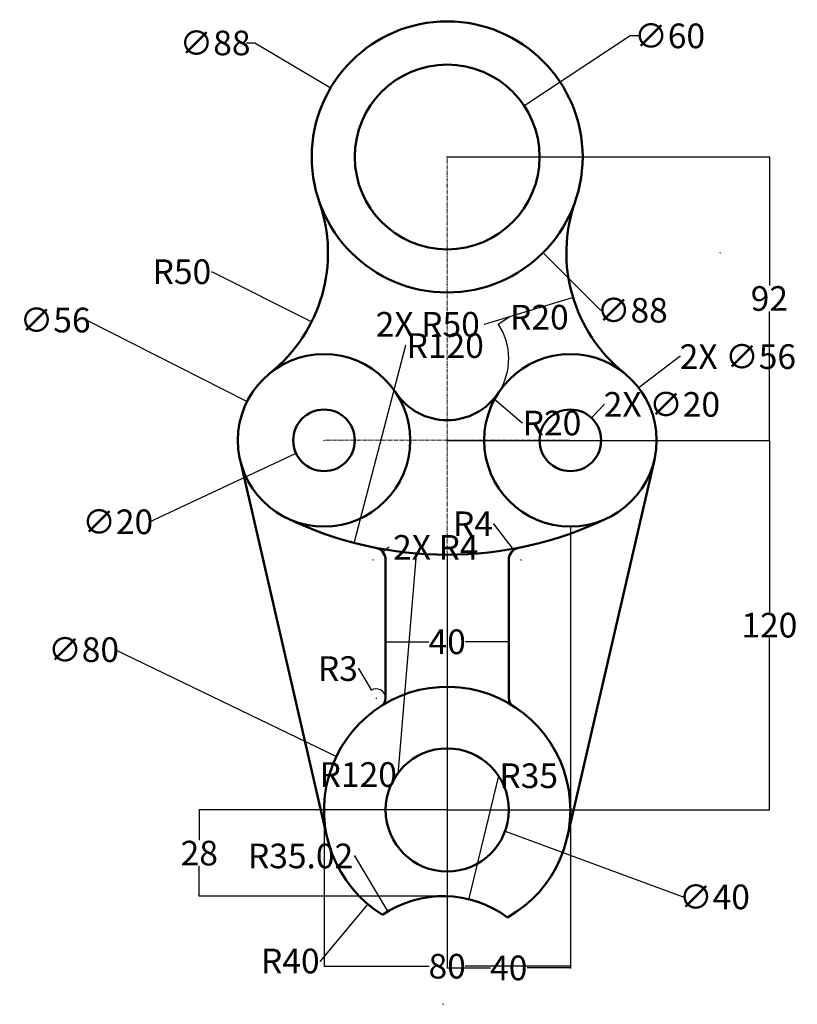
# Model space of a CAD drawing. Units: inches. Extents: x 453 to 706, y -10 to 310.
import ezdxf

# ---------------------------------------------------------------- set-up
doc = ezdxf.new("R2010")
doc.units = ezdxf.units.IN
doc.header["$MEASUREMENT"] = 0
doc.linetypes.add('CENTER', pattern=[2, 1.25, -0.25, 0.25, -0.25])
for name, color, linetype, lineweight in [('M-CNTR', 41, 'CENTER', 18), ('M-CONS', 8, 'Continuous', 13), ('M-DIMS', 131, 'Continuous', 25), ('M-OUTL', 7, 'Continuous', 50)]:
    doc.layers.add(name, color=color, linetype=linetype, lineweight=lineweight)
doc.styles.get("Standard").update_dxf_attribs({"font": 'arial.ttf'})
doc.dimstyles.new('Copy of Standard', dxfattribs={"dimtxt": 8, "dimasz": 0.18, "dimexe": 0.18, "dimexo": 0.0625, "dimgap": 0.09, "dimtad": 0, "dimtih": 1, "dimtoh": 1, "dimdec": 0, "dimzin": 0, "dimdsep": 46, "dimtxsty": 'Standard', "dimcen": 0.09, "dimadec": 0, "dimazin": 0, "dimtfac": 1, "dimtdec": 0, "dimtofl": 0, "dimtmove": 0, "dimatfit": 3, "dimfxl": 1, "dimtolj": 1, "dimtzin": 0, "dimarcsym": 0})

# ---------------------------------------------------------------- blocks, each defined once
blk = doc.blocks.new('*D1')
at = {"layer": 'Defpoints', "color": 0, "transparency": 16777216}
for p in [(554.31, 287.74), (630.03, 242.91)]:
    blk.add_point(p, dxfattribs=at)
at = {"layer": 'M-DIMS', "color": 0, "lineweight": -2, "transparency": 16777216}
for p, q in [((526.97, 302.32), (529.67, 302.32)), ((529.67, 302.32), (554.15, 287.83)), ((592.08, 265.32), (592.26, 265.32)), ((592.17, 265.23), (592.17, 265.41))]:
    blk.add_line(p, q, dxfattribs=at)
at = {"layer": 'M-DIMS', "color": 0, "transparency": 16777216}
blk.add_solid([(554.17, 287.85), (554.14, 287.8), (554.31, 287.74)], dxfattribs=at)
at = {"layer": 'M-DIMS', "color": 0, "transparency": 16777216, "insert": (516.79, 302.32), "char_height": 8, "attachment_point": 5}
blk.add_mtext('\\A1;∅88', dxfattribs=at)
blk = doc.blocks.new('*D2')
at = {"layer": 'Defpoints', "color": 0, "transparency": 16777216}
for p in [(617.19, 281.88), (567.16, 248.76)]:
    blk.add_point(p, dxfattribs=at)
at = {"layer": 'M-DIMS', "color": 0, "lineweight": -2, "transparency": 16777216}
for p, q in [((651.55, 304.63), (617.34, 281.98)), ((654.25, 304.63), (651.55, 304.63)), ((592.08, 265.32), (592.26, 265.32)), ((592.17, 265.23), (592.17, 265.41))]:
    blk.add_line(p, q, dxfattribs=at)
at = {"layer": 'M-DIMS', "color": 0, "transparency": 16777216}
blk.add_solid([(617.32, 282), (617.35, 281.95), (617.19, 281.88)], dxfattribs=at)
at = {"layer": 'M-DIMS', "color": 0, "transparency": 16777216, "insert": (664.41, 304.63), "char_height": 8, "attachment_point": 5}
blk.add_mtext('\\A1;∅60', dxfattribs=at)
blk = doc.blocks.new('*D3')
at = {"layer": 'Defpoints', "color": 0, "transparency": 16777216}
for p in [(503.46, 234.24), (548.18, 211.87)]:
    blk.add_point(p, dxfattribs=at)
at = {"layer": 'M-DIMS', "color": 0, "lineweight": -2, "transparency": 16777216}
for p, q in [((515.64, 228.06), (515.82, 228.06)), ((515.82, 228.06), (548.02, 211.95))]:
    blk.add_line(p, q, dxfattribs=at)
at = {"layer": 'M-DIMS', "color": 0, "transparency": 16777216}
blk.add_solid([(548.03, 211.98), (548, 211.93), (548.18, 211.87)], dxfattribs=at)
at = {"layer": 'M-DIMS', "color": 0, "transparency": 16777216, "insert": (506.01, 228.06), "char_height": 8, "attachment_point": 5}
blk.add_mtext('\\A1;R50', dxfattribs=at)
blk = doc.blocks.new('*D4')
at = {"layer": 'Defpoints', "color": 0, "transparency": 16777216}
for p in [(592.17, 256.17), (561.94, 140.04)]:
    blk.add_point(p, dxfattribs=at)
at = {"layer": 'M-DIMS', "color": 0, "lineweight": -2, "transparency": 16777216}
for p, q in [((578.61, 204.07), (561.99, 140.22)), ((578.79, 204.07), (578.61, 204.07))]:
    blk.add_line(p, q, dxfattribs=at)
at = {"layer": 'M-DIMS', "color": 0, "transparency": 16777216}
blk.add_solid([(561.96, 140.22), (562.01, 140.21), (561.94, 140.04)], dxfattribs=at)
at = {"layer": 'M-DIMS', "color": 0, "transparency": 16777216, "insert": (591.53, 204.07), "char_height": 8, "attachment_point": 5}
blk.add_mtext('\\A1;R120', dxfattribs=at)
blk = doc.blocks.new('*D5')
at = {"layer": 'Defpoints', "color": 0, "transparency": 16777216}
for p in [(608.81, 210.96), (592.17, 199.85)]:
    blk.add_point(p, dxfattribs=at)
at = {"layer": 'M-DIMS', "color": 0, "lineweight": -2, "transparency": 16777216}
for p, q in [((612.31, 213.3), (608.96, 211.06)), ((612.49, 213.3), (612.31, 213.3)), ((592.08, 199.85), (592.26, 199.85)), ((592.17, 199.76), (592.17, 199.94))]:
    blk.add_line(p, q, dxfattribs=at)
blk.add_arc((592.17, 199.85), 20, 326.6217, 34.236, dxfattribs=at)
at = {"layer": 'M-DIMS', "color": 0, "transparency": 16777216}
blk.add_solid([(608.94, 211.08), (608.97, 211.03), (608.81, 210.96)], dxfattribs=at)
at = {"layer": 'M-DIMS', "color": 0, "transparency": 16777216, "insert": (622.12, 213.3), "char_height": 8, "attachment_point": 5}
blk.add_mtext('\\A1;R20', dxfattribs=at)
blk = doc.blocks.new('*D6')
at = {"layer": 'Defpoints', "color": 0, "transparency": 16777216}
for p in [(592.17, 265.41), (592.17, 173.32), (696.8, 173.32)]:
    blk.add_point(p, dxfattribs=at)
at = {"layer": 'M-DIMS', "color": 0, "lineweight": -2, "transparency": 16777216}
for p, q in [((592.23, 265.41), (696.98, 265.41)), ((696.8, 265.23), (696.8, 223.54)), ((696.8, 173.5), (696.8, 215.19)), ((592.23, 173.32), (696.98, 173.32))]:
    blk.add_line(p, q, dxfattribs=at)
at = {"layer": 'M-DIMS', "color": 0, "transparency": 16777216}
for points in [[(696.77, 265.23), (696.83, 265.23), (696.8, 265.41)], [(696.77, 173.5), (696.83, 173.5), (696.8, 173.32)]]:
    blk.add_solid(points, dxfattribs=at)
at = {"layer": 'M-DIMS', "color": 0, "transparency": 16777216, "insert": (696.8, 219.37), "char_height": 8, "attachment_point": 5}
blk.add_mtext('\\A1;92', dxfattribs=at)
blk = doc.blocks.new('*D7')
at = {"layer": 'Defpoints', "color": 0, "transparency": 16777216}
for p in [(592.17, 173.32), (696.8, 173.32), (592.17, 53.32)]:
    blk.add_point(p, dxfattribs=at)
at = {"layer": 'M-DIMS', "color": 0, "lineweight": -2, "transparency": 16777216}
for p, q in [((592.23, 173.32), (696.98, 173.32)), ((696.8, 173.14), (696.8, 117.5)), ((696.8, 53.5), (696.8, 109.15)), ((592.23, 53.32), (696.98, 53.32))]:
    blk.add_line(p, q, dxfattribs=at)
at = {"layer": 'M-DIMS', "color": 0, "transparency": 16777216}
for points in [[(696.77, 173.14), (696.83, 173.14), (696.8, 173.32)], [(696.77, 53.5), (696.83, 53.5), (696.8, 53.32)]]:
    blk.add_solid(points, dxfattribs=at)
at = {"layer": 'M-DIMS', "color": 0, "transparency": 16777216, "insert": (696.8, 113.32), "char_height": 8, "attachment_point": 5}
blk.add_mtext('\\A1;120', dxfattribs=at)
blk = doc.blocks.new('*D8')
at = {"layer": 'Defpoints', "color": 0, "transparency": 16777216}
for p in [(511.67, 53.32), (592.17, 53.32), (592.17, 25.32)]:
    blk.add_point(p, dxfattribs=at)
at = {"layer": 'M-DIMS', "color": 0, "lineweight": -2, "transparency": 16777216}
for p, q in [((592.11, 53.32), (511.49, 53.32)), ((511.67, 53.14), (511.67, 43.5)), ((511.67, 25.5), (511.67, 35.15)), ((592.11, 25.32), (511.49, 25.32))]:
    blk.add_line(p, q, dxfattribs=at)
at = {"layer": 'M-DIMS', "color": 0, "transparency": 16777216}
for points in [[(511.64, 53.14), (511.7, 53.14), (511.67, 53.32)], [(511.64, 25.5), (511.7, 25.5), (511.67, 25.32)]]:
    blk.add_solid(points, dxfattribs=at)
at = {"layer": 'M-DIMS', "color": 0, "transparency": 16777216, "insert": (511.67, 39.32), "char_height": 8, "attachment_point": 5}
blk.add_mtext('\\A1;28', dxfattribs=at)
blk = doc.blocks.new('*D9')
at = {"layer": 'Defpoints', "color": 0, "transparency": 16777216}
for p in [(561.23, 177.55), (543.11, 169.09)]:
    blk.add_point(p, dxfattribs=at)
at = {"layer": 'M-DIMS', "color": 0, "lineweight": -2, "transparency": 16777216}
for p, q in [((552.08, 173.32), (552.26, 173.32)), ((552.17, 173.23), (552.17, 173.41)), ((495.51, 146.87), (542.95, 169.02)), ((495.33, 146.87), (495.51, 146.87))]:
    blk.add_line(p, q, dxfattribs=at)
at = {"layer": 'M-DIMS', "color": 0, "transparency": 16777216}
blk.add_solid([(542.93, 169.04), (542.96, 168.99), (543.11, 169.09)], dxfattribs=at)
at = {"layer": 'M-DIMS', "color": 0, "transparency": 16777216, "insert": (485.17, 146.87), "char_height": 8, "attachment_point": 5}
blk.add_mtext('\\A1;∅20', dxfattribs=at)
blk = doc.blocks.new('*D10')
at = {"layer": 'Defpoints', "color": 0, "transparency": 16777216}
for p in [(527.2, 185.99), (577.14, 160.65)]:
    blk.add_point(p, dxfattribs=at)
at = {"layer": 'M-DIMS', "color": 0, "lineweight": -2, "transparency": 16777216}
for p, q in [((475.01, 212.37), (475.19, 212.37)), ((475.19, 212.37), (527.04, 186.07)), ((552.08, 173.32), (552.26, 173.32)), ((552.17, 173.23), (552.17, 173.41))]:
    blk.add_line(p, q, dxfattribs=at)
at = {"layer": 'M-DIMS', "color": 0, "transparency": 16777216}
blk.add_solid([(527.05, 186.1), (527.03, 186.04), (527.2, 185.99)], dxfattribs=at)
at = {"layer": 'M-DIMS', "color": 0, "transparency": 16777216, "insert": (464.85, 212.37), "char_height": 8, "attachment_point": 5}
blk.add_mtext('\\A1;∅56', dxfattribs=at)
blk = doc.blocks.new('*D11')
at = {"layer": 'Defpoints', "color": 0, "transparency": 16777216}
for p in [(556.15, 70.72), (628.19, 35.93)]:
    blk.add_point(p, dxfattribs=at)
at = {"layer": 'M-DIMS', "color": 0, "lineweight": -2, "transparency": 16777216}
for p, q in [((484.25, 105.36), (484.43, 105.36)), ((484.43, 105.36), (555.99, 70.8)), ((592.08, 53.32), (592.26, 53.32)), ((592.17, 53.23), (592.17, 53.41))]:
    blk.add_line(p, q, dxfattribs=at)
at = {"layer": 'M-DIMS', "color": 0, "transparency": 16777216}
blk.add_solid([(556, 70.82), (555.98, 70.77), (556.15, 70.72)], dxfattribs=at)
at = {"layer": 'M-DIMS', "color": 0, "transparency": 16777216, "insert": (474.09, 105.36), "char_height": 8, "attachment_point": 5}
blk.add_mtext('\\A1;∅80', dxfattribs=at)
blk = doc.blocks.new('*D12')
at = {"layer": 'Defpoints', "color": 0, "transparency": 16777216}
for p in [(573.41, 60.25), (610.93, 46.4)]:
    blk.add_point(p, dxfattribs=at)
at = {"layer": 'M-DIMS', "color": 0, "lineweight": -2, "transparency": 16777216}
for p, q in [((592.08, 53.32), (592.26, 53.32)), ((592.17, 53.23), (592.17, 53.41)), ((668.63, 25.1), (611.1, 46.33)), ((668.81, 25.1), (668.63, 25.1))]:
    blk.add_line(p, q, dxfattribs=at)
at = {"layer": 'M-DIMS', "color": 0, "transparency": 16777216}
blk.add_solid([(611.11, 46.36), (611.09, 46.3), (610.93, 46.4)], dxfattribs=at)
at = {"layer": 'M-DIMS', "color": 0, "transparency": 16777216, "insert": (678.97, 25.1), "char_height": 8, "attachment_point": 5}
blk.add_mtext('\\A1;∅40', dxfattribs=at)
blk = doc.blocks.new('*D13')
at = {"layer": 'Defpoints', "color": 0, "transparency": 16777216}
for p in [(599.12, 24.37), (590.9, -9.68)]:
    blk.add_point(p, dxfattribs=at)
at = {"layer": 'M-DIMS', "color": 0, "lineweight": -2, "transparency": 16777216}
for p, q in [((608.79, 64.44), (599.16, 24.54)), ((608.97, 64.44), (608.79, 64.44)), ((590.9, -9.77), (590.9, -9.59)), ((590.81, -9.68), (590.99, -9.68))]:
    blk.add_line(p, q, dxfattribs=at)
at = {"layer": 'M-DIMS', "color": 0, "transparency": 16777216}
blk.add_solid([(599.13, 24.55), (599.19, 24.53), (599.12, 24.37)], dxfattribs=at)
at = {"layer": 'M-DIMS', "color": 0, "transparency": 16777216, "insert": (618.65, 64.44), "char_height": 8, "attachment_point": 5}
blk.add_mtext('\\A1;R35', dxfattribs=at)
blk = doc.blocks.new('*D14')
at = {"layer": 'Defpoints', "color": 0, "transparency": 16777216}
for p in [(552.17, 53.32), (632.17, 53.32), (632.17, 2.6)]:
    blk.add_point(p, dxfattribs=at)
at = {"layer": 'M-DIMS', "color": 0, "lineweight": -2, "transparency": 16777216}
for p, q in [((552.17, 53.26), (552.17, 2.42)), ((632.17, 53.26), (632.17, 2.42)), ((552.35, 2.6), (586.36, 2.6)), ((631.99, 2.6), (597.98, 2.6))]:
    blk.add_line(p, q, dxfattribs=at)
at = {"layer": 'M-DIMS', "color": 0, "transparency": 16777216}
for points in [[(552.35, 2.63), (552.35, 2.57), (552.17, 2.6)], [(631.99, 2.63), (631.99, 2.57), (632.17, 2.6)]]:
    blk.add_solid(points, dxfattribs=at)
at = {"layer": 'M-DIMS', "color": 0, "transparency": 16777216, "insert": (592.17, 2.6), "char_height": 8, "attachment_point": 5}
blk.add_mtext('\\A1;80', dxfattribs=at)
blk = doc.blocks.new('*D15')
at = {"layer": 'Defpoints', "color": 0, "transparency": 16777216}
for p in [(572.17, 112.08), (612.17, 112.08), (612.17, 107.92)]:
    blk.add_point(p, dxfattribs=at)
at = {"layer": 'M-DIMS', "color": 0, "lineweight": -2, "transparency": 16777216}
for p, q in [((572.17, 112.02), (572.17, 107.74)), ((612.17, 112.02), (612.17, 107.74)), ((572.35, 107.92), (586.2, 107.92)), ((611.99, 107.92), (598.14, 107.92))]:
    blk.add_line(p, q, dxfattribs=at)
at = {"layer": 'M-DIMS', "color": 0, "transparency": 16777216}
for points in [[(572.35, 107.95), (572.35, 107.89), (572.17, 107.92)], [(611.99, 107.95), (611.99, 107.89), (612.17, 107.92)]]:
    blk.add_solid(points, dxfattribs=at)
at = {"layer": 'M-DIMS', "color": 0, "transparency": 16777216, "insert": (592.17, 107.92), "char_height": 8, "attachment_point": 5}
blk.add_mtext('\\A1;40', dxfattribs=at)
blk = doc.blocks.new('*D16')
at = {"layer": 'Defpoints', "color": 0, "transparency": 16777216}
for p in [(613.75, 137.7), (616.17, 134.52)]:
    blk.add_point(p, dxfattribs=at)
at = {"layer": 'M-DIMS', "color": 0, "lineweight": -2, "transparency": 16777216}
for p, q in [((607.06, 146.22), (607.24, 146.22)), ((607.24, 146.22), (613.64, 137.84)), ((616.08, 134.52), (616.26, 134.52)), ((616.17, 134.43), (616.17, 134.61))]:
    blk.add_line(p, q, dxfattribs=at)
at = {"layer": 'M-DIMS', "color": 0, "transparency": 16777216}
blk.add_solid([(613.66, 137.86), (613.61, 137.82), (613.75, 137.7)], dxfattribs=at)
at = {"layer": 'M-DIMS', "color": 0, "transparency": 16777216, "insert": (600.54, 146.22), "char_height": 8, "attachment_point": 5}
blk.add_mtext('\\A1;R4', dxfattribs=at)
blk = doc.blocks.new('*D17')
at = {"layer": 'Defpoints', "color": 0, "transparency": 16777216}
for p in [(567.62, 92.22), (569.17, 89.65)]:
    blk.add_point(p, dxfattribs=at)
at = {"layer": 'M-DIMS', "color": 0, "lineweight": -2, "transparency": 16777216}
for p, q in [((563.21, 99.22), (563.39, 99.22)), ((563.39, 99.22), (567.53, 92.37)), ((569.08, 89.65), (569.26, 89.65)), ((569.17, 89.56), (569.17, 89.74))]:
    blk.add_line(p, q, dxfattribs=at)
blk.add_arc((569.17, 89.65), 3, 1.1937, 124.5815, dxfattribs=at)
at = {"layer": 'M-DIMS', "color": 0, "transparency": 16777216}
blk.add_solid([(567.55, 92.39), (567.5, 92.36), (567.62, 92.22)], dxfattribs=at)
at = {"layer": 'M-DIMS', "color": 0, "transparency": 16777216, "insert": (556.67, 99.22), "char_height": 8, "attachment_point": 5}
blk.add_mtext('\\A1;R3', dxfattribs=at)
blk = doc.blocks.new('ROLLER-BOSS-56-BORE-20')
for radius in [28, 10]:
    blk.add_circle((0, 0), radius)
blk = doc.blocks.new('*D19')
at = {"layer": 'Defpoints', "color": 0, "transparency": 16777216}
for p in [(632.17, 145.32), (592.17, 136.17), (632.17, 2.05)]:
    blk.add_point(p, dxfattribs=at)
at = {"layer": 'M-DIMS', "color": 0, "lineweight": -2, "transparency": 16777216}
for p, q in [((632.17, 145.26), (632.17, 1.87)), ((592.17, 136.11), (592.17, 1.87)), ((592.35, 2.05), (606.2, 2.05)), ((631.99, 2.05), (618.14, 2.05))]:
    blk.add_line(p, q, dxfattribs=at)
at = {"layer": 'M-DIMS', "color": 0, "transparency": 16777216}
for points in [[(592.35, 2.08), (592.35, 2.02), (592.17, 2.05)], [(631.99, 2.08), (631.99, 2.02), (632.17, 2.05)]]:
    blk.add_solid(points, dxfattribs=at)
at = {"layer": 'M-DIMS', "color": 0, "transparency": 16777216, "insert": (612.17, 2.05), "char_height": 8, "attachment_point": 5}
blk.add_mtext('\\A1;40', dxfattribs=at)
blk = doc.blocks.new('*D20')
at = {"layer": 'Defpoints', "color": 0, "transparency": 16777216}
for p in [(680.88, 234.24), (633.04, 219.71)]:
    blk.add_point(p, dxfattribs=at)
at = {"layer": 'M-DIMS', "color": 0, "lineweight": -2, "transparency": 16777216}
for p, q in [((680.79, 234.24), (680.97, 234.24)), ((680.88, 234.15), (680.88, 234.33)), ((604.34, 210.99), (632.87, 219.66)), ((604.16, 210.99), (604.34, 210.99))]:
    blk.add_line(p, q, dxfattribs=at)
at = {"layer": 'M-DIMS', "color": 0, "transparency": 16777216}
blk.add_solid([(632.86, 219.69), (632.88, 219.63), (633.04, 219.71)], dxfattribs=at)
at = {"layer": 'M-DIMS', "color": 0, "transparency": 16777216, "insert": (585.86, 210.99), "char_height": 8, "attachment_point": 5}
blk.add_mtext('\\A1;2X R50', dxfattribs=at)
blk = doc.blocks.new('*D21')
at = {"layer": 'Defpoints', "color": 0, "transparency": 16777216}
for p in [(561.06, 296.44), (623.28, 234.21)]:
    blk.add_point(p, dxfattribs=at)
at = {"layer": 'M-DIMS', "color": 0, "lineweight": -2, "transparency": 16777216}
for p, q in [((592.08, 265.32), (592.26, 265.32)), ((592.17, 265.23), (592.17, 265.41)), ((641.95, 215.54), (623.41, 234.08)), ((642.13, 215.54), (641.95, 215.54))]:
    blk.add_line(p, q, dxfattribs=at)
at = {"layer": 'M-DIMS', "color": 0, "transparency": 16777216}
blk.add_solid([(623.43, 234.1), (623.39, 234.06), (623.28, 234.21)], dxfattribs=at)
at = {"layer": 'M-DIMS', "color": 0, "transparency": 16777216, "insert": (652.31, 215.54), "char_height": 8, "attachment_point": 5}
blk.add_mtext('\\A1;∅88', dxfattribs=at)
blk = doc.blocks.new('*D22')
at = {"layer": 'Defpoints', "color": 0, "transparency": 16777216}
for p in [(592.17, 199.85), (607.31, 186.79)]:
    blk.add_point(p, dxfattribs=at)
at = {"layer": 'M-DIMS', "color": 0, "lineweight": -2, "transparency": 16777216}
for p, q in [((592.08, 199.85), (592.26, 199.85)), ((592.17, 199.76), (592.17, 199.94)), ((616.4, 178.95), (607.45, 186.67)), ((616.58, 178.95), (616.4, 178.95))]:
    blk.add_line(p, q, dxfattribs=at)
at = {"layer": 'M-DIMS', "color": 0, "transparency": 16777216}
blk.add_solid([(607.47, 186.69), (607.43, 186.65), (607.31, 186.79)], dxfattribs=at)
at = {"layer": 'M-DIMS', "color": 0, "transparency": 16777216, "insert": (626.21, 178.95), "char_height": 8, "attachment_point": 5}
blk.add_mtext('\\A1;R20', dxfattribs=at)
blk = doc.blocks.new('*D23')
at = {"layer": 'Defpoints', "color": 0, "transparency": 16777216}
for p in [(654.43, 190.31), (609.91, 156.33)]:
    blk.add_point(p, dxfattribs=at)
at = {"layer": 'M-DIMS', "color": 0, "lineweight": -2, "transparency": 16777216}
for p, q in [((667.78, 200.5), (654.57, 190.42)), ((667.96, 200.5), (667.78, 200.5)), ((632.08, 173.32), (632.26, 173.32)), ((632.17, 173.23), (632.17, 173.41))]:
    blk.add_line(p, q, dxfattribs=at)
at = {"layer": 'M-DIMS', "color": 0, "transparency": 16777216}
blk.add_solid([(654.55, 190.44), (654.59, 190.39), (654.43, 190.31)], dxfattribs=at)
at = {"layer": 'M-DIMS', "color": 0, "transparency": 16777216, "insert": (686.58, 200.5), "char_height": 8, "attachment_point": 5}
blk.add_mtext('\\A1;2X ∅56', dxfattribs=at)
blk = doc.blocks.new('*D24')
at = {"layer": 'Defpoints', "color": 0, "transparency": 16777216}
for p in [(639.01, 180.61), (625.33, 166.03)]:
    blk.add_point(p, dxfattribs=at)
at = {"layer": 'M-DIMS', "color": 0, "lineweight": -2, "transparency": 16777216}
for p, q in [((643.12, 184.99), (639.14, 180.75)), ((643.3, 184.99), (643.12, 184.99)), ((632.08, 173.32), (632.26, 173.32)), ((632.17, 173.23), (632.17, 173.41))]:
    blk.add_line(p, q, dxfattribs=at)
at = {"layer": 'M-DIMS', "color": 0, "transparency": 16777216}
blk.add_solid([(639.11, 180.77), (639.16, 180.72), (639.01, 180.61)], dxfattribs=at)
at = {"layer": 'M-DIMS', "color": 0, "transparency": 16777216, "insert": (661.91, 184.99), "char_height": 8, "attachment_point": 5}
blk.add_mtext('\\A1;2X ∅20', dxfattribs=at)
blk = doc.blocks.new('*D25')
at = {"layer": 'Defpoints', "color": 0, "transparency": 16777216}
for p in [(592.17, 256.17), (582.2, 136.59)]:
    blk.add_point(p, dxfattribs=at)
at = {"layer": 'M-DIMS', "color": 0, "lineweight": -2, "transparency": 16777216}
for p, q in [((592.08, 256.17), (592.26, 256.17)), ((592.17, 256.08), (592.17, 256.26)), ((576.22, 64.83), (582.18, 136.41)), ((576.04, 64.83), (576.22, 64.83))]:
    blk.add_line(p, q, dxfattribs=at)
at = {"layer": 'M-DIMS', "color": 0, "transparency": 16777216}
blk.add_solid([(582.15, 136.41), (582.21, 136.4), (582.2, 136.59)], dxfattribs=at)
at = {"layer": 'M-DIMS', "color": 0, "transparency": 16777216, "insert": (563.29, 64.83), "char_height": 8, "attachment_point": 5}
blk.add_mtext('\\A1;R120', dxfattribs=at)
blk = doc.blocks.new('*D26')
at = {"layer": 'Defpoints', "color": 0, "transparency": 16777216}
for p in [(568.17, 134.52), (571.26, 137.06)]:
    blk.add_point(p, dxfattribs=at)
at = {"layer": 'M-DIMS', "color": 0, "lineweight": -2, "transparency": 16777216}
for p, q in [((573.11, 138.58), (571.4, 137.17)), ((573.29, 138.58), (573.11, 138.58)), ((568.08, 134.52), (568.26, 134.52)), ((568.17, 134.43), (568.17, 134.61))]:
    blk.add_line(p, q, dxfattribs=at)
at = {"layer": 'M-DIMS', "color": 0, "transparency": 16777216}
blk.add_solid([(571.38, 137.19), (571.42, 137.15), (571.26, 137.06)], dxfattribs=at)
at = {"layer": 'M-DIMS', "color": 0, "transparency": 16777216, "insert": (588.48, 138.58), "char_height": 8, "attachment_point": 5}
blk.add_mtext('\\A1;2X R4', dxfattribs=at)
blk = doc.blocks.new('*D27')
at = {"layer": 'Defpoints', "color": 0, "transparency": 16777216}
for p in [(572.9, 20.37), (590.9, -9.68)]:
    blk.add_point(p, dxfattribs=at)
at = {"layer": 'M-DIMS', "color": 0, "lineweight": -2, "transparency": 16777216}
for p, q in [((561.92, 38.39), (562.1, 38.39)), ((562.1, 38.39), (572.81, 20.52)), ((590.9, -9.77), (590.9, -9.59)), ((590.81, -9.68), (590.99, -9.68))]:
    blk.add_line(p, q, dxfattribs=at)
at = {"layer": 'M-DIMS', "color": 0, "transparency": 16777216}
blk.add_solid([(572.83, 20.54), (572.78, 20.5), (572.9, 20.37)], dxfattribs=at)
at = {"layer": 'M-DIMS', "color": 0, "transparency": 16777216, "insert": (544.55, 38.39), "char_height": 8, "attachment_point": 5}
blk.add_mtext('\\A1;R35.02', dxfattribs=at)
blk = doc.blocks.new('*D28')
at = {"layer": 'Defpoints', "color": 0, "transparency": 16777216}
for p in [(592.17, 53.32), (566.46, 22.68)]:
    blk.add_point(p, dxfattribs=at)
at = {"layer": 'M-DIMS', "color": 0, "lineweight": -2, "transparency": 16777216}
for p, q in [((592.08, 53.32), (592.26, 53.32)), ((592.17, 53.23), (592.17, 53.41)), ((551.03, 4.29), (566.34, 22.54)), ((550.85, 4.29), (551.03, 4.29))]:
    blk.add_line(p, q, dxfattribs=at)
at = {"layer": 'M-DIMS', "color": 0, "transparency": 16777216}
blk.add_solid([(566.32, 22.56), (566.37, 22.52), (566.46, 22.68)], dxfattribs=at)
at = {"layer": 'M-DIMS', "color": 0, "transparency": 16777216, "insert": (541.22, 4.29), "char_height": 8, "attachment_point": 5}
blk.add_mtext('\\A1;R40', dxfattribs=at)

msp = doc.modelspace()

# ---------------------------------------------------------------- linework, layer by layer
at = {"layer": 'M-CNTR'}
for q in [(592.171, 265.321), (552.171, 173.321), (592.171, 53.321), (632.171, 173.321)]:
    msp.add_line((592.171, 173.321), q, dxfattribs=at)
at = {"layer": 'M-CONS'}
msp.add_line((592.171, 25.321), (589.628, 25.321), dxfattribs=at)
at = {"layer": 'M-OUTL'}
for p, q in [((553.195, 44.329), (524.888, 167.027)), ((631.148, 44.329), (659.455, 167.027)), ((572.171, 89.653), (572.171, 134.515)), ((612.171, 89.653), (612.171, 134.515)), ((612.171, 89.653), (612.171, 134.515))]:
    msp.add_line(p, q, dxfattribs=at)
for centre, radius in [((592.171, 265.321), 44), ((592.171, 265.321), 30), ((592.171, 53.321), 20)]:
    msp.add_circle(centre, radius, dxfattribs=at)
for centre, radius, start, end in [((503.459, 234.24), 50, 308.64711, 19.30845), ((680.884, 234.24), 50, 160.69155, 231.35289), ((592.171, 199.854), 20, 213.55731, 326.44269), ((592.171, 256.171), 120, 244.22854, 295.77146), ((568.171, 134.515), 4, 0, 78.84006), ((616.171, 134.515), 4, 101.15994, 180), ((592.171, 53.321), 40, 299.33247, 238.35508), ((569.171, 89.653), 3, 302.33603, 0), ((615.171, 89.653), 3, 180, 237.66397), ((590.9, -9.679), 35.023, 53.43069, 124.25686)]:
    msp.add_arc(centre, radius, start, end, dxfattribs=at)

# ---------------------------------------------------------------- block references
for p in [(552.171, 173.321), (632.171, 173.321)]:
    msp.add_blockref('ROLLER-BOSS-56-BORE-20', p, dxfattribs=at)

# ---------------------------------------------------------------- dimensions: what is measured, and where the dimension line sits
at = {"layer": 'M-DIMS'}
for p1, p2, override, picture, middle in [((630.034, 242.906), (554.309, 287.736), {"dimclrd": 0, "dimclre": 0, "dimclrt": 0}, '*D1', (516.789, 302.321)), ((567.155, 248.762), (617.187, 281.88), {"dimclrd": 0, "dimclre": 0, "dimclrt": 0}, '*D2', (664.408, 304.628)), ((561.06, 296.435), (623.283, 234.207), {"dimdec": 0, "dimlfac": 1, "dimrnd": 0, "dimzin": 0, "dimdsep": 46, "dimlunit": 2}, '*D21', (652.31, 215.539)), ((577.142, 160.653), (527.201, 185.989), {"dimclrd": 0, "dimclre": 0, "dimclrt": 0}, '*D10', (464.845, 212.373)), ((561.233, 177.551), (543.11, 169.092), {"dimclrd": 0, "dimclre": 0, "dimclrt": 0}, '*D9', (485.17, 146.872)), ((628.191, 35.925), (556.152, 70.717), {"dimclrd": 0, "dimclre": 0, "dimclrt": 0}, '*D11', (474.09, 105.358)), ((573.409, 60.247), (610.934, 46.395), {"dimclrd": 0, "dimclre": 0, "dimclrt": 0}, '*D12', (678.973, 25.096))]:
    dim = msp.add_diameter_dim_2p(p1=p1, p2=p2, dimstyle='Copy of Standard', override=override, dxfattribs=at)
    dim.commit()
    dim.dimension.update_dxf_attribs({"geometry": picture, "text_midpoint": middle, "dimtype": 163})
for base, p1, p2, picture, middle in [((696.796, 173.321), (592.171, 265.411), (592.171, 173.321), '*D6', (696.796, 219.366)), ((696.796, 173.321), (592.171, 53.321), (592.171, 173.321), '*D7', (696.796, 113.321)), ((511.666, 53.321), (592.171, 25.321), (592.171, 53.321), '*D8', (511.666, 39.321))]:
    dim = msp.add_linear_dim(base=base, p1=p1, p2=p2, angle=90, dimstyle='Copy of Standard', override={"dimclrd": 0, "dimclre": 0, "dimclrt": 0}, dxfattribs=at)
    dim.commit()
    dim.dimension.update_dxf_attribs({"geometry": picture, "text_midpoint": middle})
for center, mpoint, override, picture, middle in [((592.171, 256.171), (582.199, 136.586), {"dimdec": 0, "dimlfac": 1, "dimrnd": 0, "dimzin": 0, "dimdsep": 46, "dimlunit": 2}, '*D25', (563.293, 64.835)), ((592.171, 256.171), (561.94, 140.041), {"dimclrd": 0, "dimclre": 0, "dimclrt": 0}, '*D4', (591.531, 204.07)), ((503.459, 234.24), (548.177, 211.873), {"dimclrd": 0, "dimclre": 0, "dimclrt": 0}, '*D3', (506.007, 228.056)), ((592.171, 199.854), (608.807, 210.957), {"dimclrd": 0, "dimclre": 0, "dimclrt": 0}, '*D5', (622.125, 213.296)), ((592.171, 199.854), (607.313, 186.788), {"dimdec": 0, "dimlfac": 1, "dimrnd": 0, "dimzin": 0, "dimdsep": 46, "dimlunit": 2}, '*D22', (626.213, 178.949)), ((616.171, 134.515), (613.746, 137.696), {"dimclrd": 0, "dimclre": 0, "dimclrt": 0}, '*D16', (600.539, 146.222)), ((569.171, 89.653), (567.62, 92.221), {"dimclrd": 0, "dimclre": 0, "dimclrt": 0}, '*D17', (556.672, 99.217)), ((590.9, -9.679), (599.119, 24.366), {"dimclrd": 0, "dimclre": 0, "dimclrt": 0}, '*D13', (618.652, 64.442)), ((592.171, 53.321), (566.46, 22.68), {"dimdec": 0, "dimlfac": 1, "dimrnd": 0, "dimzin": 0, "dimdsep": 46, "dimlunit": 2}, '*D28', (541.218, 4.295)), ((590.9, -9.679), (572.901, 20.365), {"dimdec": 2, "dimlfac": 1, "dimrnd": 0, "dimzin": 0, "dimdsep": 46, "dimlunit": 2}, '*D27', (544.546, 38.392))]:
    dim = msp.add_radius_dim(center=center, mpoint=mpoint, dimstyle='Copy of Standard', override=override, dxfattribs=at)
    dim.commit()
    dim.dimension.update_dxf_attribs({"geometry": picture, "text_midpoint": middle, "dimtype": 164})
for center, mpoint, picture, middle in [((680.884, 234.24), (633.042, 219.709), '*D20', (585.86, 210.991)), ((568.171, 134.515), (571.261, 137.056), '*D26', (588.482, 138.58))]:
    dim = msp.add_radius_dim(center=center, mpoint=mpoint, text='2X <>', dimstyle='Copy of Standard', override={"dimdec": 0, "dimlfac": 1, "dimrnd": 0, "dimzin": 0, "dimdsep": 46, "dimlunit": 2}, dxfattribs=at)
    dim.commit()
    dim.dimension.update_dxf_attribs({"geometry": picture, "text_midpoint": middle, "dimtype": 164})
for p1, p2, picture, middle in [((609.914, 156.333), (654.429, 190.309), '*D23', (686.583, 200.502)), ((625.329, 166.028), (639.013, 180.614), '*D24', (661.907, 184.99))]:
    dim = msp.add_diameter_dim_2p(p1=p1, p2=p2, text='2X <>', dimstyle='Copy of Standard', override={"dimdec": 0, "dimlfac": 1, "dimrnd": 0, "dimzin": 0, "dimdsep": 46, "dimlunit": 2}, dxfattribs=at)
    dim.commit()
    dim.dimension.update_dxf_attribs({"geometry": picture, "text_midpoint": middle, "dimtype": 163})
for base, p1, p2, override, picture, middle in [((632.171, 2.05), (592.171, 136.171), (632.171, 145.321), {"dimdec": 0, "dimlfac": 1, "dimrnd": 0, "dimzin": 0, "dimdsep": 46, "dimlunit": 2}, '*D19', (612.171, 2.05)), ((612.171, 107.922), (572.171, 112.084), (612.171, 112.084), {"dimclrd": 0, "dimclre": 0, "dimclrt": 0}, '*D15', (592.171, 107.922)), ((632.171, 2.596), (552.171, 53.321), (632.171, 53.321), {"dimclrd": 0, "dimclre": 0, "dimclrt": 0}, '*D14', (592.171, 2.596))]:
    dim = msp.add_linear_dim(base=base, p1=p1, p2=p2, dimstyle='Copy of Standard', override=override, dxfattribs=at)
    dim.commit()
    dim.dimension.update_dxf_attribs({"geometry": picture, "text_midpoint": middle})

doc.saveas('drawing.dxf')
